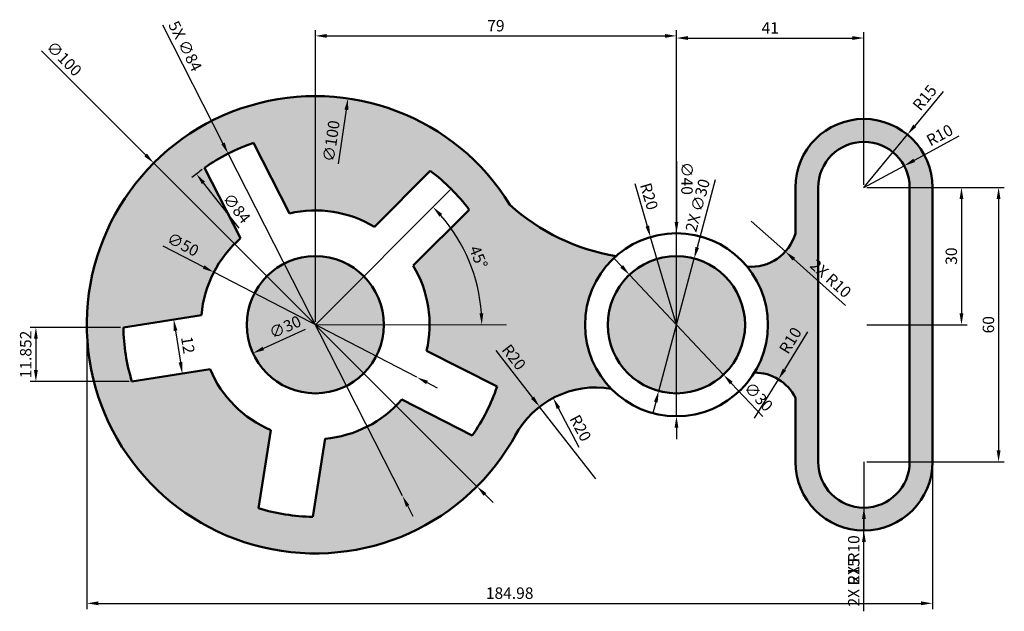
# Model space of a CAD drawing. Units: millimetres. Extents: x 2433 to 2649, y 1283 to 1412.
import ezdxf

# ---------------------------------------------------------------- set-up
doc = ezdxf.new("R2010")
doc.units = ezdxf.units.MM
for name, color, linetype, lineweight in [('M-CONS', 8, 'Continuous', 13), ('M-DIMS', 2, 'Continuous', 25), ('M-HATC', 252, 'Continuous', 18), ('M-OUTL', 7, 'Continuous', 50)]:
    doc.layers.add(name, color=color, linetype=linetype, lineweight=lineweight)
doc.styles.get("Standard").update_dxf_attribs({"font": 'arial.ttf'})
doc.dimstyles.new('ISO-25', dxfattribs={"dimtxt": 2.5, "dimasz": 2.5, "dimexe": 1.25, "dimexo": 0.625, "dimtad": 1, "dimtxsty": 'Standard', "dimcen": 2.5, "dimadec": 0, "dimazin": 0, "dimtfac": 1, "dimtmove": 0, "dimatfit": 3, "dimfxl": 1, "dimarcsym": 0})

# ---------------------------------------------------------------- blocks, each defined once
blk = doc.blocks.new('*D1')
at = {"layer": 'Defpoints', "color": 0, "transparency": 16777216}
for p in [(2576.99, 1408.65), (2497.99, 1345.49), (2576.99, 1345.49)]:
    blk.add_point(p, dxfattribs=at)
at = {"layer": 'M-DIMS', "color": 0, "lineweight": -2, "transparency": 16777216}
for p, q in [((2497.99, 1346.11), (2497.99, 1409.9)), ((2500.49, 1408.65), (2574.49, 1408.65)), ((2576.99, 1346.11), (2576.99, 1409.9))]:
    blk.add_line(p, q, dxfattribs=at)
at = {"layer": 'M-DIMS', "color": 0, "transparency": 16777216}
for points in [[(2500.49, 1409.06), (2500.49, 1408.23), (2497.99, 1408.65)], [(2574.49, 1409.06), (2574.49, 1408.23), (2576.99, 1408.65)]]:
    blk.add_solid(points, dxfattribs=at)
at = {"layer": 'M-DIMS', "color": 0, "transparency": 16777216, "insert": (2537.49, 1410.55), "char_height": 2.5, "attachment_point": 5}
blk.add_mtext('79', dxfattribs=at)
blk = doc.blocks.new('*D2')
at = {"layer": 'Defpoints', "color": 0, "transparency": 16777216}
for p in [(2617.99, 1408.18), (2617.99, 1375.49), (2576.99, 1345.49)]:
    blk.add_point(p, dxfattribs=at)
at = {"layer": 'M-DIMS', "color": 0, "lineweight": -2, "transparency": 16777216}
for p, q in [((2576.99, 1346.11), (2576.99, 1409.43)), ((2617.99, 1376.11), (2617.99, 1409.43)), ((2579.49, 1408.18), (2615.49, 1408.18))]:
    blk.add_line(p, q, dxfattribs=at)
at = {"layer": 'M-DIMS', "color": 0, "transparency": 16777216}
for points in [[(2579.49, 1408.6), (2579.49, 1407.77), (2576.99, 1408.18)], [(2615.49, 1408.6), (2615.49, 1407.77), (2617.99, 1408.18)]]:
    blk.add_solid(points, dxfattribs=at)
at = {"layer": 'M-DIMS', "color": 0, "transparency": 16777216, "insert": (2597.49, 1410.06), "char_height": 2.5, "attachment_point": 5}
blk.add_mtext('41', dxfattribs=at)
blk = doc.blocks.new('*D3')
at = {"layer": 'Defpoints', "color": 0, "transparency": 16777216}
for p in [(2617.99, 1375.49), (2617.99, 1315.49), (2647.45, 1315.49)]:
    blk.add_point(p, dxfattribs=at)
at = {"layer": 'M-DIMS', "color": 0, "lineweight": -2, "transparency": 16777216}
for p, q in [((2618.62, 1375.49), (2648.7, 1375.49)), ((2647.45, 1372.99), (2647.45, 1317.99)), ((2618.62, 1315.49), (2648.7, 1315.49))]:
    blk.add_line(p, q, dxfattribs=at)
at = {"layer": 'M-DIMS', "color": 0, "transparency": 16777216}
for points in [[(2647.03, 1372.99), (2647.87, 1372.99), (2647.45, 1375.49)], [(2647.03, 1317.99), (2647.87, 1317.99), (2647.45, 1315.49)]]:
    blk.add_solid(points, dxfattribs=at)
at = {"layer": 'M-DIMS', "color": 0, "transparency": 16777216, "insert": (2645.55, 1345.49), "char_height": 2.5, "attachment_point": 5, "rotation": 90}
blk.add_mtext('60', dxfattribs=at)
blk = doc.blocks.new('*D4')
at = {"layer": 'Defpoints', "color": 0, "transparency": 16777216}
for p in [(2617.99, 1375.49), (2617.99, 1345.49), (2639.33, 1345.49)]:
    blk.add_point(p, dxfattribs=at)
at = {"layer": 'M-DIMS', "color": 0, "lineweight": -2, "transparency": 16777216}
for p, q in [((2618.62, 1375.49), (2640.58, 1375.49)), ((2639.33, 1372.99), (2639.33, 1347.99)), ((2618.62, 1345.49), (2640.58, 1345.49))]:
    blk.add_line(p, q, dxfattribs=at)
at = {"layer": 'M-DIMS', "color": 0, "transparency": 16777216}
for points in [[(2638.91, 1372.99), (2639.75, 1372.99), (2639.33, 1375.49)], [(2638.91, 1347.99), (2639.75, 1347.99), (2639.33, 1345.49)]]:
    blk.add_solid(points, dxfattribs=at)
at = {"layer": 'M-DIMS', "color": 0, "transparency": 16777216, "insert": (2637.43, 1360.49), "char_height": 2.5, "attachment_point": 5, "rotation": 90}
blk.add_mtext('30', dxfattribs=at)
blk = doc.blocks.new('*D5')
at = {"layer": 'Defpoints', "color": 0, "transparency": 16777216}
for p in [(2527.69, 1375.18), (2533.16, 1354.91), (2497.99, 1345.49), (2497.99, 1345.49), (2539.8, 1345.49)]:
    blk.add_point(p, dxfattribs=at)
at = {"layer": 'M-DIMS', "color": 0, "lineweight": -2, "transparency": 16777216}
blk.add_arc((2497.99, 1345.49), 36.41, 3.9349, 41.0651, dxfattribs=at)
at = {"layer": 'M-DIMS', "color": 0, "transparency": 16777216}
for points in [[(2525.14, 1369.12), (2525.75, 1369.69), (2523.74, 1371.23)], [(2534.73, 1348), (2533.9, 1347.97), (2534.4, 1345.49)]]:
    blk.add_solid(points, dxfattribs=at)
at = {"layer": 'M-DIMS', "color": 0, "transparency": 16777216, "insert": (2533.38, 1360.15), "char_height": 2.5, "attachment_point": 5, "rotation": 292.5}
blk.add_mtext('45°', dxfattribs=at)
blk = doc.blocks.new('*D6')
at = {"layer": 'Defpoints', "color": 0, "transparency": 16777216}
for p in [(2627.52, 1387.07), (2617.99, 1375.49)]:
    blk.add_point(p, dxfattribs=at)
at = {"layer": 'M-DIMS', "color": 0, "lineweight": -2, "transparency": 16777216}
for p, q in [((2635.3, 1396.52), (2629.11, 1389)), ((2617.99, 1375.49), (2627.52, 1387.07))]:
    blk.add_line(p, q, dxfattribs=at)
at = {"layer": 'M-DIMS', "color": 0, "transparency": 16777216}
blk.add_solid([(2628.79, 1389.26), (2629.43, 1388.73), (2627.52, 1387.07)], dxfattribs=at)
at = {"layer": 'M-DIMS', "color": 0, "transparency": 16777216, "insert": (2631.53, 1394.93), "char_height": 2.5, "attachment_point": 5, "rotation": 50.5434}
blk.add_mtext('R15', dxfattribs=at)
blk = doc.blocks.new('*D7')
at = {"layer": 'Defpoints', "color": 0, "transparency": 16777216}
for p in [(2626.79, 1380.24), (2617.99, 1375.49)]:
    blk.add_point(p, dxfattribs=at)
at = {"layer": 'M-DIMS', "color": 0, "lineweight": -2, "transparency": 16777216}
for p, q in [((2638.79, 1386.72), (2628.99, 1381.42)), ((2617.99, 1375.49), (2626.79, 1380.24))]:
    blk.add_line(p, q, dxfattribs=at)
at = {"layer": 'M-DIMS', "color": 0, "transparency": 16777216}
blk.add_solid([(2628.79, 1381.79), (2629.19, 1381.06), (2626.79, 1380.24)], dxfattribs=at)
at = {"layer": 'M-DIMS', "color": 0, "transparency": 16777216, "insert": (2634.72, 1386.67), "char_height": 2.5, "attachment_point": 5, "rotation": 28.3596}
blk.add_mtext('R10', dxfattribs=at)
blk = doc.blocks.new('*D8')
at = {"layer": 'Defpoints', "color": 0, "transparency": 16777216}
for p in [(2599.29, 1333.55), (2594.06, 1325.03)]:
    blk.add_point(p, dxfattribs=at)
at = {"layer": 'M-DIMS', "color": 0, "lineweight": -2, "transparency": 16777216}
for p, q in [((2605.68, 1343.96), (2600.6, 1335.68)), ((2594.06, 1325.03), (2599.29, 1333.55))]:
    blk.add_line(p, q, dxfattribs=at)
at = {"layer": 'M-DIMS', "color": 0, "transparency": 16777216}
blk.add_solid([(2600.25, 1335.9), (2600.96, 1335.46), (2599.29, 1333.55)], dxfattribs=at)
at = {"layer": 'M-DIMS', "color": 0, "transparency": 16777216, "insert": (2602.17, 1341.88), "char_height": 2.5, "attachment_point": 5, "rotation": 58.4653}
blk.add_mtext('R10', dxfattribs=at)
blk = doc.blocks.new('*D9')
at = {"layer": 'Defpoints', "color": 0, "transparency": 16777216}
for p in [(2571.31, 1364.66), (2576.99, 1345.49)]:
    blk.add_point(p, dxfattribs=at)
at = {"layer": 'M-DIMS', "color": 0, "lineweight": -2, "transparency": 16777216}
for p, q in [((2567.85, 1376.38), (2570.6, 1367.06)), ((2576.99, 1345.49), (2571.31, 1364.66))]:
    blk.add_line(p, q, dxfattribs=at)
at = {"layer": 'M-DIMS', "color": 0, "transparency": 16777216}
blk.add_solid([(2571, 1367.18), (2570.2, 1366.94), (2571.31, 1364.66)], dxfattribs=at)
at = {"layer": 'M-DIMS', "color": 0, "transparency": 16777216, "insert": (2570.69, 1373.46), "char_height": 2.5, "attachment_point": 5, "rotation": 286.4906}
blk.add_mtext('R20', dxfattribs=at)
blk = doc.blocks.new('*D10')
at = {"layer": 'Defpoints', "color": 0, "transparency": 16777216}
for p in [(2550.01, 1329.47), (2559.34, 1311.78)]:
    blk.add_point(p, dxfattribs=at)
at = {"layer": 'M-DIMS', "color": 0, "lineweight": -2, "transparency": 16777216}
blk.add_line((2555.71, 1318.67), (2551.17, 1327.26), dxfattribs=at)
at = {"layer": 'M-DIMS', "color": 0, "transparency": 16777216}
blk.add_solid([(2551.54, 1327.46), (2550.8, 1327.07), (2550.01, 1329.47)], dxfattribs=at)
at = {"layer": 'M-DIMS', "color": 0, "transparency": 16777216, "insert": (2555.7, 1322.75), "char_height": 2.5, "attachment_point": 5, "rotation": 297.8088}
blk.add_mtext('R20', dxfattribs=at)
blk = doc.blocks.new('*D11')
at = {"layer": 'Defpoints', "color": 0, "transparency": 16777216}
for p in [(2505.14, 1394.97), (2490.84, 1296)]:
    blk.add_point(p, dxfattribs=at)
at = {"layer": 'M-DIMS', "color": 0, "lineweight": -2, "transparency": 16777216}
blk.add_line((2503.07, 1380.64), (2504.78, 1392.5), dxfattribs=at)
at = {"layer": 'M-DIMS', "color": 0, "transparency": 16777216}
blk.add_solid([(2504.37, 1392.56), (2505.19, 1392.44), (2505.14, 1394.97)], dxfattribs=at)
at = {"layer": 'M-DIMS', "color": 0, "transparency": 16777216, "insert": (2501.79, 1385.61), "char_height": 2.5, "attachment_point": 5, "rotation": 81.7832}
blk.add_mtext('∅100', dxfattribs=at)
blk = doc.blocks.new('*D12')
at = {"layer": 'Defpoints', "color": 0, "transparency": 16777216}
for p in [(2471.97, 1378.45), (2524.01, 1312.52)]:
    blk.add_point(p, dxfattribs=at)
at = {"layer": 'M-DIMS', "color": 0, "lineweight": -2, "transparency": 16777216}
blk.add_line((2481.33, 1366.59), (2473.52, 1376.49), dxfattribs=at)
blk.add_arc((2497.99, 1345.49), 42, 126.0658, 129.9934, dxfattribs=at)
at = {"layer": 'M-DIMS', "color": 0, "transparency": 16777216}
blk.add_solid([(2473.84, 1376.75), (2473.19, 1376.23), (2471.97, 1378.45)], dxfattribs=at)
at = {"layer": 'M-DIMS', "color": 0, "transparency": 16777216, "insert": (2480.54, 1370.77), "char_height": 2.5, "attachment_point": 5, "rotation": 308.2881}
blk.add_mtext('∅84', dxfattribs=at)
blk = doc.blocks.new('*D13')
at = {"layer": 'Defpoints', "color": 0, "transparency": 16777216}
for p in [(2475.78, 1356.97), (2520.2, 1334)]:
    blk.add_point(p, dxfattribs=at)
at = {"layer": 'M-DIMS', "color": 0, "lineweight": -2, "transparency": 16777216}
for p, q in [((2464.64, 1362.73), (2473.56, 1358.12)), ((2520.2, 1334), (2475.78, 1356.97)), ((2522.42, 1332.86), (2524.64, 1331.71))]:
    blk.add_line(p, q, dxfattribs=at)
at = {"layer": 'M-DIMS', "color": 0, "transparency": 16777216}
for points in [[(2473.75, 1358.49), (2473.37, 1357.75), (2475.78, 1356.97)], [(2522.61, 1333.23), (2522.23, 1332.49), (2520.2, 1334)]]:
    blk.add_solid(points, dxfattribs=at)
at = {"layer": 'M-DIMS', "color": 0, "transparency": 16777216, "insert": (2468.9, 1362.75), "char_height": 2.5, "attachment_point": 5, "rotation": 332.6594}
blk.add_mtext('∅50', dxfattribs=at)
blk = doc.blocks.new('*D14')
at = {"layer": 'Defpoints', "color": 0, "transparency": 16777216}
for p in [(2511.64, 1351.71), (2484.34, 1339.26)]:
    blk.add_point(p, dxfattribs=at)
at = {"layer": 'M-DIMS', "color": 0, "lineweight": -2, "transparency": 16777216}
blk.add_line((2495.75, 1344.47), (2486.62, 1340.3), dxfattribs=at)
at = {"layer": 'M-DIMS', "color": 0, "transparency": 16777216}
blk.add_solid([(2486.44, 1340.68), (2486.79, 1339.92), (2484.34, 1339.26)], dxfattribs=at)
at = {"layer": 'M-DIMS', "color": 0, "transparency": 16777216, "insert": (2491.51, 1344.7), "char_height": 2.5, "attachment_point": 5, "rotation": 24.513}
blk.add_mtext('∅30', dxfattribs=at)
blk = doc.blocks.new('*D15')
at = {"layer": 'Defpoints', "color": 0, "transparency": 16777216}
for p in [(2566.71, 1356.41), (2587.27, 1334.56)]:
    blk.add_point(p, dxfattribs=at)
at = {"layer": 'M-DIMS', "color": 0, "lineweight": -2, "transparency": 16777216}
for p, q in [((2565, 1358.23), (2563.28, 1360.05)), ((2566.71, 1356.41), (2587.27, 1334.56)), ((2595.87, 1325.43), (2588.98, 1332.74))]:
    blk.add_line(p, q, dxfattribs=at)
at = {"layer": 'M-DIMS', "color": 0, "transparency": 16777216}
for points in [[(2565.3, 1358.52), (2564.69, 1357.95), (2566.71, 1356.41)], [(2589.29, 1333.03), (2588.68, 1332.46), (2587.27, 1334.56)]]:
    blk.add_solid(points, dxfattribs=at)
at = {"layer": 'M-DIMS', "color": 0, "transparency": 16777216, "insert": (2594.72, 1329.53), "char_height": 2.5, "attachment_point": 5, "rotation": 313.2584}
blk.add_mtext('∅30', dxfattribs=at)
blk = doc.blocks.new('DISC-RADIAL-SLOT-12')
for p, q in [((25.15, 33.64), (12.92, 21.4)), ((33.64, 25.15), (21.4, 12.92))]:
    blk.add_line(p, q)
blk.add_arc((0, 0), 42, 36.7868, 53.2132)
blk = doc.blocks.new('*D17')
at = {"layer": 'Defpoints', "color": 0, "transparency": 16777216}
for p in [(2455.99, 1344.91), (2468.88, 1334.8), (2457.87, 1333.06)]:
    blk.add_point(p, dxfattribs=at)
at = {"layer": 'M-DIMS', "color": 0, "lineweight": -2, "transparency": 16777216}
for p, q in [((2456.61, 1345.01), (2468.24, 1346.85)), ((2467.4, 1344.18), (2468.49, 1337.27)), ((2458.49, 1333.15), (2470.12, 1335))]:
    blk.add_line(p, q, dxfattribs=at)
at = {"layer": 'M-DIMS', "color": 0, "transparency": 16777216}
for points in [[(2467.81, 1344.25), (2466.99, 1344.12), (2467.01, 1346.65)], [(2468.9, 1337.34), (2468.08, 1337.21), (2468.88, 1334.8)]]:
    blk.add_solid(points, dxfattribs=at)
at = {"layer": 'M-DIMS', "color": 0, "transparency": 16777216, "insert": (2469.8, 1341.02), "char_height": 2.5, "attachment_point": 5, "rotation": 279}
blk.add_mtext('12', dxfattribs=at)
blk = doc.blocks.new('*D18')
at = {"layer": 'Defpoints', "color": 0, "transparency": 16777216}
for p in [(2448.01, 1344.05), (2632.99, 1315.49), (2632.99, 1284.57)]:
    blk.add_point(p, dxfattribs=at)
at = {"layer": 'M-DIMS', "color": 0, "lineweight": -2, "transparency": 16777216}
for p, q in [((2448.01, 1343.42), (2448.01, 1283.32)), ((2632.99, 1314.86), (2632.99, 1283.32)), ((2450.51, 1284.57), (2630.49, 1284.57))]:
    blk.add_line(p, q, dxfattribs=at)
at = {"layer": 'M-DIMS', "color": 0, "transparency": 16777216}
for points in [[(2450.51, 1284.99), (2450.51, 1284.16), (2448.01, 1284.57)], [(2630.49, 1284.99), (2630.49, 1284.16), (2632.99, 1284.57)]]:
    blk.add_solid(points, dxfattribs=at)
at = {"layer": 'M-DIMS', "color": 0, "transparency": 16777216, "insert": (2540.5, 1286.47), "char_height": 2.5, "attachment_point": 5}
blk.add_mtext('184.98', dxfattribs=at)
blk = doc.blocks.new('*D19')
at = {"layer": 'Defpoints', "color": 0, "transparency": 16777216}
for p in [(2455.99, 1344.91), (2436.86, 1333.06), (2457.87, 1333.06)]:
    blk.add_point(p, dxfattribs=at)
at = {"layer": 'M-DIMS', "color": 0, "lineweight": -2, "transparency": 16777216}
for p, q in [((2455.37, 1344.91), (2435.61, 1344.91)), ((2436.86, 1342.41), (2436.86, 1335.56)), ((2457.25, 1333.06), (2435.61, 1333.06))]:
    blk.add_line(p, q, dxfattribs=at)
at = {"layer": 'M-DIMS', "color": 0, "transparency": 16777216}
for points in [[(2436.44, 1342.41), (2437.28, 1342.41), (2436.86, 1344.91)], [(2436.44, 1335.56), (2437.28, 1335.56), (2436.86, 1333.06)]]:
    blk.add_solid(points, dxfattribs=at)
at = {"layer": 'M-DIMS', "color": 0, "transparency": 16777216, "insert": (2434.96, 1338.98), "char_height": 2.5, "attachment_point": 5, "rotation": 90}
blk.add_mtext('11.852', dxfattribs=at)
blk = doc.blocks.new('*D20')
at = {"layer": 'Defpoints', "color": 0, "transparency": 16777216}
for p in [(2462.64, 1380.84), (2533.34, 1310.13)]:
    blk.add_point(p, dxfattribs=at)
at = {"layer": 'M-DIMS', "color": 0, "lineweight": -2, "transparency": 16777216}
for p, q in [((2438.07, 1405.41), (2460.87, 1382.61)), ((2533.34, 1310.13), (2462.64, 1380.84)), ((2535.11, 1308.36), (2536.88, 1306.59))]:
    blk.add_line(p, q, dxfattribs=at)
at = {"layer": 'M-DIMS', "color": 0, "transparency": 16777216}
for points in [[(2461.16, 1382.91), (2460.57, 1382.32), (2462.64, 1380.84)], [(2535.41, 1308.66), (2534.82, 1308.07), (2533.34, 1310.13)]]:
    blk.add_solid(points, dxfattribs=at)
at = {"layer": 'M-DIMS', "color": 0, "transparency": 16777216, "insert": (2442.82, 1403.45), "char_height": 2.5, "attachment_point": 5, "rotation": 314.9971}
blk.add_mtext('∅100', dxfattribs=at)
blk = doc.blocks.new('*D21')
at = {"layer": 'Defpoints', "color": 0, "transparency": 16777216}
for p in [(2478.92, 1382.91), (2517.06, 1308.06)]:
    blk.add_point(p, dxfattribs=at)
at = {"layer": 'M-DIMS', "color": 0, "lineweight": -2, "transparency": 16777216}
for p, q in [((2464.58, 1411.06), (2477.79, 1385.14)), ((2517.06, 1308.06), (2478.92, 1382.91)), ((2518.19, 1305.84), (2519.33, 1303.61))]:
    blk.add_line(p, q, dxfattribs=at)
at = {"layer": 'M-DIMS', "color": 0, "transparency": 16777216}
for points in [[(2478.16, 1385.33), (2477.42, 1384.95), (2478.92, 1382.91)], [(2518.56, 1306.03), (2517.82, 1305.65), (2517.06, 1308.06)]]:
    blk.add_solid(points, dxfattribs=at)
at = {"layer": 'M-DIMS', "color": 0, "transparency": 16777216, "insert": (2469.24, 1406.26), "char_height": 2.5, "attachment_point": 5, "rotation": 296.9999}
blk.add_mtext('5X ∅84', dxfattribs=at)
blk = doc.blocks.new('*D22')
at = {"layer": 'Defpoints', "color": 0, "transparency": 16777216}
for p in [(2580.87, 1359.98), (2573.11, 1331)]:
    blk.add_point(p, dxfattribs=at)
at = {"layer": 'M-DIMS', "color": 0, "lineweight": -2, "transparency": 16777216}
for p, q in [((2585.48, 1377.19), (2581.52, 1362.39)), ((2573.11, 1331), (2580.87, 1359.98)), ((2572.46, 1328.58), (2571.81, 1326.17))]:
    blk.add_line(p, q, dxfattribs=at)
at = {"layer": 'M-DIMS', "color": 0, "transparency": 16777216}
for points in [[(2581.12, 1362.5), (2581.92, 1362.28), (2580.87, 1359.98)], [(2572.06, 1328.69), (2572.86, 1328.47), (2573.11, 1331)]]:
    blk.add_solid(points, dxfattribs=at)
at = {"layer": 'M-DIMS', "color": 0, "transparency": 16777216, "insert": (2581.92, 1371.51), "char_height": 2.5, "attachment_point": 5, "rotation": 75.0022}
blk.add_mtext('2X ∅30', dxfattribs=at)
blk = doc.blocks.new('*D23')
at = {"layer": 'Defpoints', "color": 0, "transparency": 16777216}
for p in [(2576.99, 1365.49), (2576.99, 1325.49)]:
    blk.add_point(p, dxfattribs=at)
at = {"layer": 'M-DIMS', "color": 0, "lineweight": -2, "transparency": 16777216}
for p, q in [((2576.99, 1381.26), (2576.99, 1367.99)), ((2576.99, 1325.49), (2576.99, 1365.49)), ((2576.99, 1322.99), (2576.99, 1320.49))]:
    blk.add_line(p, q, dxfattribs=at)
at = {"layer": 'M-DIMS', "color": 0, "transparency": 16777216}
for points in [[(2577.41, 1367.99), (2576.57, 1367.99), (2576.99, 1365.49)], [(2577.41, 1322.99), (2576.57, 1322.99), (2576.99, 1325.49)]]:
    blk.add_solid(points, dxfattribs=at)
at = {"layer": 'M-DIMS', "color": 0, "transparency": 16777216, "insert": (2578.96, 1377.49), "char_height": 2.5, "attachment_point": 5, "rotation": 270.0009}
blk.add_mtext('∅40', dxfattribs=at)
blk = doc.blocks.new('*D24')
at = {"layer": 'Defpoints', "color": 0, "transparency": 16777216}
for p in [(2547.05, 1327.56), (2559.34, 1311.78)]:
    blk.add_point(p, dxfattribs=at)
at = {"layer": 'M-DIMS', "color": 0, "lineweight": -2, "transparency": 16777216}
for p, q in [((2537.46, 1339.88), (2545.51, 1329.54)), ((2559.34, 1311.78), (2547.05, 1327.56))]:
    blk.add_line(p, q, dxfattribs=at)
at = {"layer": 'M-DIMS', "color": 0, "transparency": 16777216}
blk.add_solid([(2545.84, 1329.79), (2545.19, 1329.28), (2547.05, 1327.56)], dxfattribs=at)
at = {"layer": 'M-DIMS', "color": 0, "transparency": 16777216, "insert": (2541.18, 1338.2), "char_height": 2.5, "attachment_point": 5, "rotation": 307.9021}
blk.add_mtext('R20', dxfattribs=at)
blk = doc.blocks.new('*D25')
at = {"layer": 'Defpoints', "color": 0, "transparency": 16777216}
for p in [(2593.36, 1368.16), (2600.81, 1361.49)]:
    blk.add_point(p, dxfattribs=at)
at = {"layer": 'M-DIMS', "color": 0, "lineweight": -2, "transparency": 16777216}
for p, q in [((2593.36, 1368.16), (2600.81, 1361.49)), ((2613.94, 1349.73), (2602.67, 1359.82))]:
    blk.add_line(p, q, dxfattribs=at)
at = {"layer": 'M-DIMS', "color": 0, "transparency": 16777216}
blk.add_solid([(2602.95, 1360.13), (2602.39, 1359.51), (2600.81, 1361.49)], dxfattribs=at)
at = {"layer": 'M-DIMS', "color": 0, "transparency": 16777216, "insert": (2610.51, 1355.36), "char_height": 2.5, "attachment_point": 5, "rotation": 318.1497}
blk.add_mtext('2X R10', dxfattribs=at)
blk = doc.blocks.new('*D26')
at = {"layer": 'Defpoints', "color": 0, "transparency": 16777216}
for p in [(2617.99, 1315.49), (2617.99, 1305.49)]:
    blk.add_point(p, dxfattribs=at)
at = {"layer": 'M-DIMS', "color": 0, "lineweight": -2, "transparency": 16777216}
for p, q in [((2617.99, 1315.49), (2617.99, 1305.49)), ((2617.99, 1287.86), (2617.99, 1302.99))]:
    blk.add_line(p, q, dxfattribs=at)
at = {"layer": 'M-DIMS', "color": 0, "transparency": 16777216}
blk.add_solid([(2617.57, 1302.99), (2618.41, 1302.99), (2617.99, 1305.49)], dxfattribs=at)
at = {"layer": 'M-DIMS', "color": 0, "transparency": 16777216, "insert": (2616.09, 1294.17), "char_height": 2.5, "attachment_point": 5, "rotation": 89.9982}
blk.add_mtext('2X R10', dxfattribs=at)
blk = doc.blocks.new('*D27')
at = {"layer": 'Defpoints', "color": 0, "transparency": 16777216}
for p in [(2617.99, 1315.49), (2617.99, 1300.49)]:
    blk.add_point(p, dxfattribs=at)
at = {"layer": 'M-DIMS', "color": 0, "lineweight": -2, "transparency": 16777216}
for p, q in [((2617.99, 1315.49), (2617.99, 1300.49)), ((2617.99, 1282.83), (2617.99, 1297.99))]:
    blk.add_line(p, q, dxfattribs=at)
at = {"layer": 'M-DIMS', "color": 0, "transparency": 16777216}
blk.add_solid([(2617.57, 1297.99), (2618.41, 1297.99), (2617.99, 1300.49)], dxfattribs=at)
at = {"layer": 'M-DIMS', "color": 0, "transparency": 16777216, "insert": (2616.09, 1289.16), "char_height": 2.5, "attachment_point": 5, "rotation": 89.9988}
blk.add_mtext('2X R15', dxfattribs=at)

msp = doc.modelspace()

# ---------------------------------------------------------------- hatches: boundary and pattern name
at = {"layer": 'M-HATC'}
h = msp.add_hatch(color=256, dxfattribs=at)
h.set_gradient(color1=(0, 255, 255), color2=(0, 255, 0), tint=1)
h.paths.add_polyline_path([(2632.9903, 1375.4861, 1), (2602.9903, 1375.4861), (2602.9903, 1365.4698, -0.36273569), (2592.4226, 1358.2079, -0.17408161), (2596.9903, 1345.4861, -0.13847123), (2594.0368, 1335.0258, -0.28376902), (2602.9903, 1329.5316), (2602.9903, 1315.4861, 1), (2632.9903, 1315.4861)])
h.paths.add_polyline_path([(2607.9903, 1375.4861, -1), (2627.9903, 1375.4861), (2627.9903, 1315.4861, -1), (2607.9903, 1315.4861)], flags=16)
h.paths.add_polyline_path([(2541.6338, 1321.0884, -0.32462061), (2562.6955, 1331.4983, -0.19609346), (2556.9903, 1345.4861, -0.21568459), (2563.7865, 1360.5081, -0.14645502), (2540.5472, 1371.7333, 3.67613447)])
h.paths.add_polyline_path([(2500.1199, 1320.577), (2497.4136, 1303.4901, -0.07179677), (2485.5613, 1305.3673), (2488.2676, 1322.4542, -0.19540804), (2474.9584, 1335.7634), (2457.8715, 1333.0571, -0.07179677), (2455.9943, 1344.9094), (2473.0812, 1347.6157, -0.19540804), (2481.6262, 1364.3863), (2473.7722, 1379.8006, -0.07179677), (2484.4643, 1385.2485), (2492.3183, 1369.8342, -0.19540804), (2510.9087, 1366.8898), (2523.1416, 1379.1226, -0.07179677), (2531.6268, 1370.6374), (2519.394, 1358.4045, -0.19540804), (2522.3384, 1339.8141), (2537.7527, 1331.9601, -0.07179677), (2532.3048, 1321.2681), (2516.8905, 1329.122, -0.19540804)], flags=16)
h.paths.add_polyline_path([(2482.9903, 1345.4861, -1), (2512.9903, 1345.4861, -1)], flags=0)
h.paths.add_polyline_path([(2602.359, 1337.2119), (2606.3637, 1343.738), (2601.9727, 1346.4325), (2597.9681, 1339.9064)], flags=24)
h.paths.add_polyline_path([(2529.7699, 1362.0829), (2532.2694, 1356.0487), (2537.029, 1358.0202), (2534.5295, 1364.0544)], flags=24)
h.paths.add_polyline_path([(2503.6788, 1380.4051), (2505.0785, 1390.0982), (2499.9796, 1390.8345), (2498.5799, 1381.1414)], flags=24)
h.paths.add_polyline_path([(2476.0717, 1372.2196), (2480.9365, 1366.0571), (2484.9801, 1369.2493), (2480.1153, 1375.4118)], flags=24)
h.paths.add_polyline_path([(2464.2221, 1362.2256), (2471.1963, 1358.6197), (2473.5624, 1363.196), (2466.5882, 1366.8019)], flags=24)
h.paths.add_polyline_path([(2489.0282, 1340.6965), (2496.1718, 1343.954), (2494.0344, 1348.6415), (2486.8907, 1345.384)], flags=8)
h = msp.add_hatch(color=256, dxfattribs=at)
h.set_gradient(color1=(255, 255, 255), color2=(255, 0, 255), tint=1, name='INVSPHERICAL')
h.paths.add_polyline_path([(2508.5969, 1356.0927), (2497.9903, 1345.4861), (2512.9903, 1345.4861, 0.19891237)], flags=17)
h.paths.add_polyline_path([(2508.5969, 1356.0927, 0.66817864), (2482.9903, 1345.4861, 1), (2512.9903, 1345.4861), (2497.9903, 1345.4861)])
h.paths.add_polyline_path([(2591.9903, 1345.4861, 1), (2561.9903, 1345.4861, 1)])

# ---------------------------------------------------------------- linework, layer by layer
at = {"layer": 'M-CONS'}
for p, q in [((2516.4833, 1372.4644), (2523.1416, 1379.1226)), ((2497.9903, 1345.4861), (2527.6888, 1375.1846)), ((2524.9686, 1363.9791), (2531.6268, 1370.6374)), ((2497.9903, 1345.4861), (2539.7971, 1345.4861))]:
    msp.add_line(p, q, dxfattribs=at)
at = {"layer": 'M-OUTL'}
for p, q in [((2602.9903, 1375.4861), (2602.9903, 1365.4698)), ((2607.9903, 1375.4861), (2607.9903, 1315.4861)), ((2627.9903, 1375.4861), (2627.9903, 1315.4861)), ((2632.9903, 1375.4861), (2632.9903, 1315.4861)), ((2602.9903, 1329.5316), (2602.9903, 1315.4861))]:
    msp.add_line(p, q, dxfattribs=at)
for centre, radius in [((2576.9903, 1345.4861), 20), ((2497.9903, 1345.4861), 15), ((2576.9903, 1345.4861), 15)]:
    msp.add_circle(centre, radius, dxfattribs=at)
for centre, radius, start, end in [((2497.9903, 1345.4861), 50, 31.664418, 331.63737), ((2617.9903, 1375.4861), 15, 0, 180), ((2617.9903, 1375.4861), 10, 0, 180), ((2497.9903, 1345.4861), 25, 58.88654, 103.11346), ((2570.9174, 1404.9395), 45, 227.554122, 260.882202), ((2497.9903, 1345.4861), 25, 130.88654, 175.11346), ((2593.36, 1368.1639), 10, 264.621246, 344.371306), ((2497.9903, 1345.4861), 25, 346.88654, 31.11346), ((2497.9903, 1345.4861), 25, 202.88654, 247.11346), ((2594.0629, 1325.0259), 10, 26.780665, 90.149863), ((2559.3368, 1311.7823), 20, 80.3321, 152.270095), ((2497.9903, 1345.4861), 25, 274.88654, 319.11346), ((2617.9903, 1315.4861), 15, 180, 0), ((2617.9903, 1315.4861), 10, 180, 0)]:
    msp.add_arc(centre, radius, start, end, dxfattribs=at)

# ---------------------------------------------------------------- block references
for rotation in [72.00000000000142, 144.0000000000012, 288.0000000000003, 215.9999999999996]:
    msp.add_blockref('DISC-RADIAL-SLOT-12', (2497.9903, 1345.4861), dxfattribs=dict(at, rotation=rotation))
msp.add_blockref('DISC-RADIAL-SLOT-12', (2497.9903, 1345.4861), dxfattribs=at)

# ---------------------------------------------------------------- dimensions: what is measured, and where the dimension line sits
at = {"layer": 'M-DIMS'}
for p1, p2, text, picture, middle in [((2517.0579, 1308.0638), (2478.9228, 1382.9084), '5X <>', '*D21', (2467.4823, 1405.3618)), ((2573.1086, 1330.9971), (2580.872, 1359.9752), '2X <>', '*D22', (2583.8253, 1370.9984))]:
    dim = msp.add_diameter_dim_2p(p1=p1, p2=p2, text=text, dimstyle='ISO-25', override={"dimdec": 0, "dimlfac": 1, "dimrnd": 0, "dimzin": 0, "dimdsep": 46, "dimlunit": 2}, dxfattribs=at)
    dim.commit()
    dim.dimension.update_dxf_attribs({"geometry": picture, "text_midpoint": middle, "dimtype": 163})
for base, p1, p2, override, picture, middle in [((2576.9903, 1408.6468), (2497.9903, 1345.4861), (2576.9903, 1345.4861), {"dimclrd": 0, "dimclre": 0, "dimclrt": 0}, '*D1', (2537.4903, 1410.5482)), ((2617.9903, 1408.1831), (2576.9903, 1345.4861), (2617.9903, 1375.4861), {"dimclrd": 0, "dimclre": 0, "dimclrt": 0}, '*D2', (2597.4903, 1410.0632)), ((2632.9903, 1284.573), (2448.0111, 1344.0457), (2632.9903, 1315.4861), {"dimdec": 2, "dimlfac": 1, "dimrnd": 0, "dimzin": 0, "dimdsep": 46, "dimlunit": 2}, '*D18', (2540.5007, 1286.4745))]:
    dim = msp.add_linear_dim(base=base, p1=p1, p2=p2, dimstyle='ISO-25', override=override, dxfattribs=at)
    dim.commit()
    dim.dimension.update_dxf_attribs({"geometry": picture, "text_midpoint": middle})
for p1, p2, override, picture, middle in [((2533.3439, 1310.129), (2462.6368, 1380.8432), {"dimdec": 0, "dimlfac": 1, "dimrnd": 0, "dimzin": 0, "dimdsep": 46, "dimlunit": 2}, '*D20', (2441.4246, 1402.0575)), ((2490.8443, 1295.9994), (2505.1363, 1394.9728), {"dimclrd": 0, "dimclre": 0, "dimclrt": 0}, '*D11', (2503.7439, 1385.3304)), ((2576.9906, 1325.4861), (2576.99, 1365.4861), {"dimdec": 0, "dimlfac": 1, "dimrnd": 0, "dimzin": 0, "dimdsep": 46, "dimlunit": 2}, '*D23', (2576.9898, 1377.4861)), ((2524.0142, 1312.5201), (2471.9664, 1378.4521), {"dimclrd": 0, "dimclre": 0, "dimclrt": 0}, '*D12', (2478.9976, 1369.5453)), ((2511.6383, 1351.7096), (2484.3423, 1339.2626), {"dimclrd": 0, "dimclre": 0, "dimclrt": 0}, '*D14', (2492.323, 1342.9018))]:
    dim = msp.add_diameter_dim_2p(p1=p1, p2=p2, dimstyle='ISO-25', override=override, dxfattribs=at)
    dim.commit()
    dim.dimension.update_dxf_attribs({"geometry": picture, "text_midpoint": middle, "dimtype": 163})
for center, mpoint, picture, middle in [((2617.9903, 1375.4861), (2627.5227, 1387.0677), '*D6', (2631.5333, 1394.9326)), ((2576.9903, 1345.4861), (2571.3132, 1364.6635), '*D9', (2570.6931, 1373.4567)), ((2594.0629, 1325.0259), (2599.2931, 1333.5491), '*D8', (2602.1744, 1341.88))]:
    dim = msp.add_radius_dim(center=center, mpoint=mpoint, dimstyle='ISO-25', override={"dimclrd": 0, "dimclre": 0, "dimclrt": 0}, dxfattribs=at)
    dim.commit()
    dim.dimension.update_dxf_attribs({"geometry": picture, "text_midpoint": middle})
for center, mpoint, override, picture, middle in [((2617.9903, 1375.4861), (2626.7902, 1380.2362), {"dimclrd": 0, "dimclre": 0, "dimclrt": 0}, '*D7', (2635.6187, 1385.0017)), ((2559.3368, 1311.7823), (2547.0505, 1327.5636), {"dimdec": 0, "dimlfac": 1, "dimrnd": 0, "dimzin": 0, "dimdsep": 46, "dimlunit": 2}, '*D24', (2539.6787, 1337.0323)), ((2559.3368, 1311.7823), (2550.0064, 1329.4725), {"dimclrd": 0, "dimclre": 0, "dimclrt": 0}, '*D10', (2554.022, 1321.859))]:
    dim = msp.add_radius_dim(center=center, mpoint=mpoint, dimstyle='ISO-25', override=override, dxfattribs=at)
    dim.commit()
    dim.dimension.update_dxf_attribs({"geometry": picture, "text_midpoint": middle, "dimtype": 164})
dim = msp.add_angular_dim_2l(base=(2533.159, 1354.9095), line1=((2497.9903, 1345.4861), (2527.6888, 1375.1846)), line2=((2497.9903, 1345.4861), (2539.7971, 1345.4861)), dimstyle='ISO-25', override={"dimclrd": 0, "dimclre": 0, "dimclrt": 0}, dxfattribs=at)
dim.commit()
dim.dimension.update_dxf_attribs({"geometry": '*D5', "text_midpoint": (2533.3801, 1360.1451)})
for base, p1, p2, angle, override, picture, middle in [((2647.4514, 1315.4861), (2617.9903, 1375.4861), (2617.9903, 1315.4861), 90, {"dimclrd": 0, "dimclre": 0, "dimclrt": 0}, '*D3', (2645.5499, 1345.4861)), ((2639.3309, 1345.4861), (2617.9903, 1375.4861), (2617.9903, 1345.4861), 90, {"dimclrd": 0, "dimclre": 0, "dimclrt": 0}, '*D4', (2637.4286, 1360.4861)), ((2468.8842, 1334.8014), (2455.9943, 1344.9094), (2457.8715, 1333.0571), 279, {"dimdec": 0, "dimlfac": 1, "dimrnd": 0, "dimzin": 0, "dimdsep": 46, "dimlunit": 2}, '*D17', (2469.8026, 1341.0216)), ((2436.8611, 1333.0571), (2455.9943, 1344.9094), (2457.8715, 1333.0571), 90, {"dimdec": 3, "dimlfac": 1, "dimrnd": 0, "dimzin": 0, "dimdsep": 46, "dimlunit": 2}, '*D19', (2434.9596, 1338.9833))]:
    dim = msp.add_linear_dim(base=base, p1=p1, p2=p2, angle=angle, dimstyle='ISO-25', override=override, dxfattribs=at)
    dim.commit()
    dim.dimension.update_dxf_attribs({"geometry": picture, "text_midpoint": middle})
for center, mpoint, picture, middle in [((2593.36, 1368.1639), (2600.8089, 1361.492), '*D25', (2610.5058, 1355.3593)), ((2617.9903, 1315.4861), (2617.99, 1305.4861), '*D26', (2616.0882, 1294.1714)), ((2617.9903, 1315.4861), (2617.99, 1300.4861), '*D27', (2616.0883, 1289.1577))]:
    dim = msp.add_radius_dim(center=center, mpoint=mpoint, text='2X <>', dimstyle='ISO-25', override={"dimdec": 0, "dimlfac": 1, "dimrnd": 0, "dimzin": 0, "dimdsep": 46, "dimlunit": 2}, dxfattribs=at)
    dim.commit()
    dim.dimension.update_dxf_attribs({"geometry": picture, "text_midpoint": middle})
for p1, p2, picture, middle in [((2520.1976, 1334.0042), (2475.783, 1356.9681), '*D13', (2468.8969, 1362.7477)), ((2566.711, 1356.4102), (2587.2697, 1334.5621), '*D15', (2594.7162, 1329.5251))]:
    dim = msp.add_diameter_dim_2p(p1=p1, p2=p2, dimstyle='ISO-25', override={"dimclrd": 0, "dimclre": 0, "dimclrt": 0}, dxfattribs=at)
    dim.commit()
    dim.dimension.update_dxf_attribs({"geometry": picture, "text_midpoint": middle})

doc.saveas('drawing.dxf')
